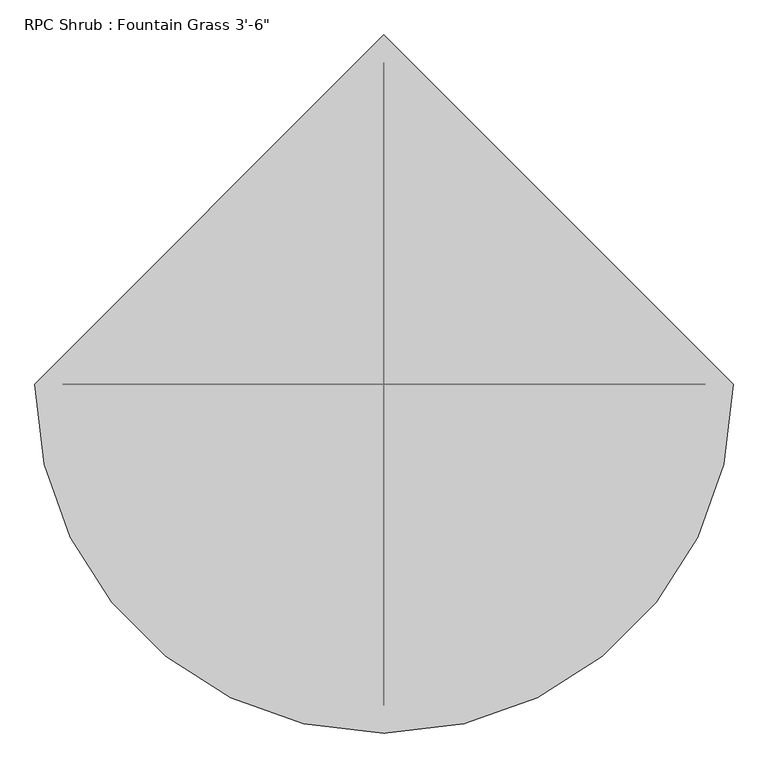
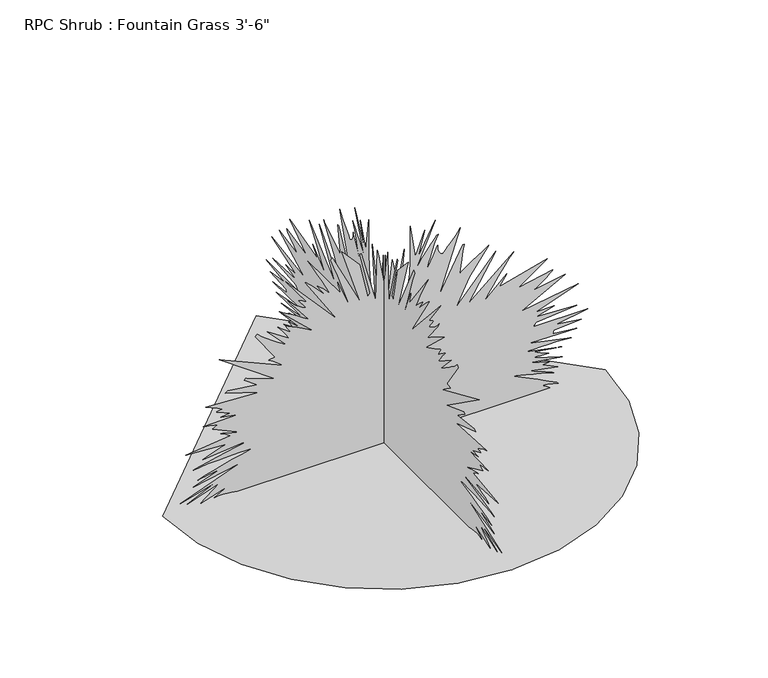
"""IFC4 building model written with IfcOpenShell, lengths in millimetres: geographic element geometry."""

from ifc_helpers import new_model, si_unit, origin, place, context, project, spatial, triangles, source, transform, mapped, element, save


def geographic_element_3d6ded1d(model_context):
    return source(origin(), model_context, "Body", "Tessellation", [
        triangles([(-1075.1021822, 0.0, 0.0), (-1046.6796438, -246.3421583, 0.0), (-965.7324045, -472.5690837, 0.0), (-838.7452429, -672.1950891, 0.0), (-672.1950891, -838.7452429, 0.0), (-472.5690837, -965.7324045, 0.0), (-246.341904, -1046.6796438, 0.0), (4.7e-05, -1075.1021822, 0.0), (246.3421583, -1046.6796438, 0.0), (472.5690837, -965.7324045, 0.0), (672.1950891, -838.7452429, 0.0), (838.7452429, -672.1950891, 0.0), (965.7324045, -472.5690837, 0.0), (1046.6796438, -246.341904, 0.0), (1075.1021822, 9.4e-05, 0.0), (-0.000141, 1075.1021822, 0.0), (-0.0002094, 151.7493584, 903.5253731), (-0.0002064, 197.8505688, 1023.5783649), (-0.0002098, 163.2745906, 893.9190554), (-0.000206, 247.7932689, 1057.1952084), (-0.0002115, 151.7493584, 831.4910345), (-0.0002109, 167.7051159, 857.3634378), (-0.0002104, 186.8993659, 885.4837418), (-0.0002098, 207.3806375, 913.5837708), (-0.0002093, 227.1984504, 939.3926605), (-0.0002089, 244.4013429, 960.6372213), (-0.0002086, 257.0401245, 975.0516758), (-0.0002085, 263.1615169, 980.3602907), (-0.0002094, 247.7267213, 943.5176268), (-0.0002103, 234.4486256, 908.2090988), (-0.0002111, 223.4664289, 876.1391087), (-0.0002118, 214.9206206, 848.9967247), (-0.0002123, 208.9511085, 828.4836599), (-0.0002127, 205.6989088, 816.294215), (-0.0002127, 205.3039292, 814.1250887), (-0.0002127, 208.3029104, 818.0239786), (-0.0002124, 216.0537091, 832.5501995), (-0.000212, 226.6881618, 853.6500017), (-0.0002116, 238.3378685, 877.271961), (-0.0002112, 249.1338665, 899.3648712), (-0.0002109, 257.207756, 915.8748373), (-0.0002107, 260.692645, 922.748037), (-0.0002103, 260.2582965, 906.3549242), (-0.0002103, 263.0522939, 893.568568), (-0.0002106, 267.949415, 883.9953152), (-0.0002111, 273.8345936, 877.2388962), (-0.0002116, 279.5876763, 872.9031143), (-0.000212, 284.0860209, 870.5917728), (-0.0002121, 286.2119994, 869.908457), (-0.0002118, 297.8807457, 886.1644415), (-0.0002115, 309.7933362, 900.0811066), (-0.0002113, 321.8837319, 912.8293837), (-0.0002111, 334.0884012, 925.5801315), (-0.0002109, 346.3388163, 939.504427), (-0.0002105, 358.5765141, 955.7731287), (-0.0002101, 370.7304234, 975.5571682), (-0.0002182, 267.0019983, 658.6111799), (-0.000213, 382.2543929, 884.3153538), (-0.0002131, 389.9378629, 884.3153538), (-0.0002137, 385.7570498, 861.6865025), (-0.0002144, 381.2002785, 835.410272), (-0.0002152, 376.6689054, 808.0824343), (-0.0002159, 372.5719171, 782.3039932), (-0.0002165, 369.305474, 760.6733368), (-0.0002169, 367.2760194, 745.7889982), (-0.0002171, 366.8873803, 740.2492201), (-0.0002169, 377.1819918, 749.4998909), (-0.0002168, 398.429096, 764.5798571), (-0.0002166, 426.0591682, 782.8856438), (-0.0002164, 455.5053723, 801.8137035), (-0.0002163, 482.19564, 818.763105), (-0.0002161, 501.5631351, 831.122743), (-0.0002161, 509.0332824, 836.294157), (-0.0002187, 412.9883454, 706.6349201), (-0.0002218, 347.6799408, 572.1725244), (-0.0002178, 543.6077345, 793.0735394), (-0.0002226, 409.1478822, 572.1725244), (-0.0002221, 630.0006443, 760.9578398), (-0.0002225, 607.1482965, 733.4877869), (-0.0002229, 581.7076618, 698.9640947), (-0.0002232, 555.6879564, 661.3112331), (-0.0002235, 531.0982146, 624.4456781), (-0.0002238, 509.9451453, 592.2867763), (-0.000224, 494.2377829, 568.7536923), (-0.0002241, 485.9827998, 557.7656639), (-0.0002226, 597.394713, 658.6111799), (-0.0002236, 558.9747108, 605.7868607), (-0.0002249, 793.3225067, 668.217425), (-0.000226, 651.1791481, 567.3694018), (-0.0002272, 820.215996, 600.9862453), (-0.0002273, 814.2901949, 595.3652584), (-0.0002274, 803.8635057, 586.2314046), (-0.0002276, 790.0737951, 574.7607748), (-0.0002278, 774.0693214, 562.1243005), (-0.0002279, 756.9878059, 549.4928767), (-0.000228, 739.9748909, 538.045138), (-0.0002281, 724.171059, 528.951943), (-0.0002293, 881.683901, 557.7656639), (-0.0002299, 666.5461607, 442.5132874), (-0.0002323, 943.1518787, 485.7338688), (-0.0002317, 735.6975357, 413.6995302), (-0.0002329, 827.8994659, 413.6995302), (-0.0002325, 739.5380716, 389.6889682), (-0.0002353, 935.4683361, 380.0852303), (-0.0002333, 739.5380716, 360.875211), (-0.0002334, 737.0615513, 358.3860097), (-0.0002334, 734.2345436, 355.2567312), (-0.0002335, 731.3236748, 351.8201314), (-0.0002335, 728.5931728, 348.4089297), (-0.0002336, 726.3148235, 345.3558457), (-0.0002336, 724.7527096, 342.9987222), (-0.0002337, 724.171059, 341.6677714), (-0.0002372, 989.2528439, 341.6677714), (-0.0002359, 835.5829359, 317.6571731), (-0.0002381, 958.5188187, 298.4471538), (-0.0002366, 824.0564592, 288.843434), (-0.000237, 820.215996, 274.4365736), (-0.0002389, 935.4683361, 260.0296949), (-0.0002357, 704.9635832, 264.8328356), (-0.0002397, 908.5748468, 221.6119818), (-0.0002392, 879.3065025, 224.4689658), (-0.0002387, 841.8263048, 226.3310433), (-0.0002381, 800.7671831, 227.3607588), (-0.0002376, 760.7622849, 227.7214381), (-0.0002371, 726.4494083, 227.5753896), (-0.0002368, 702.461701, 227.0854304), (-0.0002367, 693.4371065, 226.4143594), (-0.0002399, 862.4738817, 192.7990239), (-0.0002375, 720.3305958, 212.0077533), (-0.0002395, 801.079664, 180.0418811), (-0.0002393, 789.8198135, 180.8544223), (-0.0002391, 775.0700598, 181.8744909), (-0.0002389, 758.976638, 182.9049694), (-0.0002386, 743.6934866, 183.7490131), (-0.0002385, 731.3642973, 184.2100133), (-0.0002384, 724.1406103, 184.090889), (-0.0002384, 724.171059, 183.194523), (-0.0002416, 866.3169611, 139.9746865), (-0.0002388, 708.8040464, 163.9857935), (-0.0002409, 802.8830423, 135.5523002), (-0.0002408, 799.4514931, 134.831959), (-0.0002408, 794.1606823, 134.0915427), (-0.0002407, 787.8817778, 133.3391994), (-0.0002407, 781.4835491, 132.5827867), (-0.0002406, 775.8346207, 131.8306978), (-0.0002406, 771.8087036, 131.0902815), (-0.0002406, 770.2720242, 130.3701946), (-0.0002426, 843.2664785, 96.75485), (-0.0002398, 697.2953739, 122.86552), (-0.0002401, 707.9455233, 119.2147799), (-0.0002406, 727.4654074, 112.0362392), (-0.0002412, 752.0246641, 102.744419), (-0.0002418, 777.7954748, 92.7543584), (-0.0002424, 800.9424631, 83.4810781), (-0.0002428, 817.6404264, 76.3393719), (-0.000243, 824.0564592, 72.7440018), (-0.0002423, 793.2310152, 81.617738), (-0.0002416, 757.9402914, 91.2158803), (-0.0002408, 721.5396063, 100.7012479), (-0.0002401, 687.3868217, 109.2361467), (-0.0002395, 658.8372562, 115.9836545), (-0.0002392, 639.2462282, 120.1060682), (-0.000239, 631.9691288, 120.7659571), (-0.00024, 666.4089598, 103.8820858), (-0.0002411, 705.799288, 84.5753155), (-0.0002422, 746.4087278, 64.5205076), (-0.0002433, 784.498554, 45.3925509), (-0.0002442, 816.3297506, 28.8660546), (-0.0002449, 838.1686792, 16.6156986), (-0.0002452, 846.2788673, 10.3164533), (-0.0002449, 834.4653442, 14.1385651), (-0.0002446, 820.7849293, 17.3725156), (-0.0002444, 806.5482256, 20.018432), (-0.0002441, 793.0684525, 22.0761847), (-0.0002439, 781.6562857, 23.5461577), (-0.0002438, 773.6197123, 24.4280193), (-0.0002437, 770.2720242, 24.7219217), (-0.0002438, 772.6468792, 22.8719915), (-0.000244, 777.9732983, 19.2397436), (-0.0002442, 785.103023, 14.5784422), (-0.0002445, 792.8881582, 9.6414491), (-0.0002447, 800.1804457, 5.1824076), (-0.0002449, 805.8319902, 1.9544036), (-0.000245, 808.6894466, 0.7109504), (-0.0002248, -712.2762182, 7.55e-05), (-0.0002247, -716.251339, 1.888295), (-0.0002245, -727.0437761, 4.4398649), (-0.0002242, -742.9644613, 7.0367071), (-0.0002239, -762.3193119, 9.0605264), (-0.0002236, -783.416498, 9.8934675), (-0.0002233, -804.5594662, 8.9170168), (-0.0002232, -824.0564592, 5.5131917), (-0.0002229, -758.7480183, 43.9307805), (-0.0002224, -893.2079069, 0.7110012), (-0.0002215, -801.0059767, 72.7440018), (-0.000221, -954.6783554, 19.9198029), (-0.000221, -820.215996, 82.3482439), (-0.0002201, -989.2528439, 34.3262887), (-0.0002208, -701.1205765, 139.9746865), (-0.0002191, -927.7848661, 96.75485), (-0.0002194, -808.6894466, 139.9746865), (-0.0002193, -812.3292681, 139.9878942), (-0.0002192, -822.1235104, 138.9035673), (-0.0002191, -836.3982931, 136.9663127), (-0.000219, -853.4747217, 134.4199656), (-0.0002188, -871.6762997, 131.5086244), (-0.0002187, -889.3216616, 128.4766238), (-0.0002185, -904.7343836, 125.5680804), (-0.0002186, -893.5940025, 129.4418265), (-0.0002187, -867.1881289, 137.4656826), (-0.0002189, -829.5479118, 148.2962261), (-0.0002191, -784.7068262, 160.5885445), (-0.0002194, -736.7034336, 172.9992332), (-0.0002196, -689.5686653, 184.1843608), (-0.0002199, -647.3361414, 192.7990239), (-0.0002198, -647.3361414, 197.6011291), (-0.0002195, -670.2748575, 197.8660475), (-0.000219, -707.9862185, 197.3700022), (-0.0002184, -755.0320387, 196.1048178), (-0.0002178, -805.9742054, 194.0624097), (-0.0002172, -855.3746058, 191.2351477), (-0.0002168, -897.79004, 187.6151289), (-0.0002165, -927.7848661, 183.194523), (-0.0002165, -918.4681383, 186.3568118), (-0.0002167, -893.3831142, 192.5249491), (-0.0002169, -856.8325836, 200.7720656), (-0.0002172, -813.1090897, 210.171837), (-0.0002176, -766.5153494, 219.7974123), (-0.0002179, -721.3516817, 228.7219402), (-0.0002182, -681.9131006, 236.0185879), (-0.0002181, -681.9131006, 240.8209655), (-0.000216, -881.683901, 221.6119818), (-0.000216, -877.2592438, 223.6533724), (-0.000216, -864.5567488, 228.9396232), (-0.000216, -846.1366522, 236.2129074), (-0.0002161, -824.5568647, 244.2159255), (-0.0002161, -802.3750065, 251.6913958), (-0.0002162, -782.1465174, 257.3830178), (-0.0002164, -766.4315609, 260.0296949), (-0.0002133, -962.3618254, 274.4365736), (-0.0002155, -747.2215416, 298.4471538), (-0.0002154, -748.9690367, 300.212453), (-0.0002152, -753.6680231, 303.7532252), (-0.000215, -760.5209478, 308.3607565), (-0.0002147, -768.7124537, 313.3315287), (-0.0002145, -777.4449875, 317.9594075), (-0.0002143, -785.9107498, 321.5357517), (-0.0002141, -793.3021591, 323.3569342), (-0.0002142, -787.9021254, 322.9682951), (-0.0002145, -773.9448378, 319.7958507), (-0.0002149, -754.7907017, 314.8758748), (-0.0002153, -733.8001951, 309.2421344), (-0.0002157, -714.3387377, 303.9360992), (-0.0002161, -699.7641912, 299.9914817), (-0.0002162, -693.4371065, 298.4471538), (-0.0002125, -831.7399292, 360.875211), (-0.0002125, -830.7239302, 362.5795401), (-0.0002124, -827.9833271, 364.8223901), (-0.0002124, -823.9904022, 367.3496704), (-0.0002124, -819.2127142, 369.9125227), (-0.0002124, -814.1174583, 372.2544219), (-0.0002124, -809.1745914, 374.1289078), (-0.0002124, -804.8489834, 375.2820714), (-0.0002124, -807.681078, 376.3869822), (-0.0002122, -815.2883898, 378.2437366), (-0.000212, -826.3196205, 380.5906863), (-0.0002117, -839.4361164, 383.168763), (-0.0002115, -853.2892679, 385.7163909), (-0.0002112, -866.5404213, 387.9770087), (-0.000211, -877.8408943, 389.6889682), (-0.0002131, -712.6470531, 394.4920907), (-0.0002116, -793.3225067, 408.8989511), (-0.0002121, -743.3810783, 413.6995302), (-0.0002103, -812.5324533, 442.5132874), (-0.0002103, -811.3640654, 443.8569191), (-0.0002103, -808.2246494, 445.132023), (-0.0002103, -803.6476032, 446.2470712), (-0.0002104, -798.178969, 447.1106812), (-0.0002104, -792.3547606, 447.6364486), (-0.0002105, -786.7133898, 447.7354978), (-0.0002106, -781.7985008, 447.31641), (-0.0002105, -785.3392731, 449.5770278), (-0.0002102, -794.7525066, 454.4588882), (-0.0002098, -808.222106, 461.0349403), (-0.0002094, -823.9294321, 468.375517), (-0.000209, -840.0584621, 475.5561107), (-0.0002086, -854.7929552, 481.6521049), (-0.0002083, -866.3169611, 485.7338688), (-0.0002122, -605.078183, 471.3270083), (-0.0002084, -770.2720242, 524.1513276), (-0.0002083, -758.7480183, 533.7550655), (-0.0002108, -616.6021889, 514.5450826), (-0.0002087, -678.0700939, 557.7656639), (-0.0002085, -670.386624, 567.3694018), (-0.0002119, -528.2407219, 514.5450826), (-0.0002026, -801.0059767, 706.6349201), (-0.0002107, -493.6662698, 572.1725244), (-0.0002103, -502.7518707, 579.84077), (-0.0002099, -513.8160936, 588.6494983), (-0.0002095, -525.7210719, 597.7502872), (-0.0002091, -537.32883, 606.3024905), (-0.0002087, -547.4989941, 613.4576134), (-0.0002085, -555.0935886, 618.3700315), (-0.0002084, -558.9772542, 620.1936848), (-0.0002084, -557.3414892, 621.3672323), (-0.0002084, -553.1149303, 622.2358566), (-0.0002085, -547.2958088, 622.8886511), (-0.0002085, -540.8924569, 623.4067881), (-0.0002086, -534.9133161, 623.8742014), (-0.0002086, -530.3616317, 624.3770777), (-0.0002086, -528.2407219, 624.99688), (-0.0002032, -624.2856588, 764.2598185), (-0.000203, -616.6021889, 773.8661362), (-0.0002039, -593.2849711, 753.716276), (-0.0002049, -567.5725871, 733.8154558), (-0.0002058, -541.6163589, 715.1616526), (-0.0002066, -517.5625946, 698.7558226), (-0.0002072, -497.5601091, 685.596088), (-0.0002077, -483.7552105, 676.68326), (-0.0002079, -478.2992935, 673.0180767), (-0.0002038, -566.6607242, 769.062941), (-0.0002074, -459.0893106, 697.0286751), (-0.0002072, -461.8096387, 701.9384771), (-0.0002069, -466.5873631, 709.5711508), (-0.0002066, -473.2904423, 719.5050648), (-0.0002061, -481.786726, 731.3211313), (-0.0002056, -491.9467163, 744.6002626), (-0.000205, -503.6332486, 758.9207548), (-0.0002044, -516.7167523, 773.8661362), (-0.0002045, -513.2318996, 772.2836746), (-0.0002048, -504.2098123, 766.0124004), (-0.0002052, -491.8044648, 756.8075117), (-0.0002057, -478.1697593, 746.4290754), (-0.0002062, -465.4570905, 736.6373766), (-0.0002065, -455.8177806, 729.1875406), (-0.0002067, -451.4058043, 725.842396), (-0.0002064, -455.2462675, 731.5675552), (-0.0002062, -459.8665524, 738.7150841), (-0.0002059, -464.8017526, 746.5230377), (-0.0002056, -469.5794769, 754.2243118), (-0.0002053, -473.7349282, 761.0594324), (-0.0002051, -476.7956062, 766.2588243), (-0.000205, -478.2992935, 769.062941), (-0.0002053, -467.4382559, 763.1752916), (-0.0002059, -448.0021966, 753.3581583), (-0.0002066, -423.3616948, 740.947724), (-0.0002073, -396.8746124, 727.2876566), (-0.0002081, -371.9089851, 713.7214788), (-0.0002087, -351.8277617, 701.5879171), (-0.0002091, -339.9964345, 692.2280233), (-0.0002022, -509.0332824, 850.7010538), (-0.0002024, -501.3497761, 846.621797), (-0.000203, -481.4362023, 834.9479456), (-0.0002039, -453.9940547, 818.4430664), (-0.0002048, -423.7299863, 799.8731243), (-0.0002057, -395.3480704, 782.0093164), (-0.0002064, -373.5523441, 767.6151369), (-0.0002068, -363.0469171, 759.4592394), (-0.0002065, -368.546, 766.7414257), (-0.0002058, -383.526917, 785.5628059), (-0.0002047, -404.1618493, 811.3869564), (-0.0002036, -426.6281379, 839.67491), (-0.0002025, -447.1030509, 865.8851561), (-0.0002018, -461.7588424, 885.4786549), (-0.0002014, -466.7727805, 893.9190554), (-0.0002023, -448.2638449, 874.4677717), (-0.000203, -430.4813184, 858.5800787), (-0.0002036, -414.1669072, 846.0858559), (-0.000204, -400.0597741, 836.8173809), (-0.0002044, -388.9066395, 830.6070768), (-0.0002046, -381.4441226, 827.2873667), (-0.0002046, -378.4138933, 826.687912), (-0.0002027, -412.9883454, 874.7116522), (-0.0002028, -410.1994168, 874.6379648), (-0.0002029, -404.7105077, 872.2808413), (-0.0002031, -397.603565, 868.4733702), (-0.0002034, -389.9581741, 864.0537998), (-0.0002036, -382.8487244, 859.8627766), (-0.0002037, -377.3623587, 856.730991), (-0.0002038, -374.5708866, 855.5016329), (-0.0001983, -478.2992935, 994.7671148), (-0.0002099, -228.5847938, 716.2386217), (-0.0002007, -382.2543929, 956.3471489), (-0.0002008, -377.5401458, 953.682704), (-0.0002013, -366.727361, 944.1653343), (-0.0002019, -351.5610629, 929.5552523), (-0.0002027, -333.7912173, 911.6203005), (-0.0002035, -315.1705153, 892.1258509), (-0.0002043, -297.4463973, 872.8294996), (-0.000205, -282.3689745, 855.5016329), (-0.0002026, -324.6294582, 917.9296537), (-0.0002027, -320.6416566, 916.0831095), (-0.000203, -312.1021706, 909.1260487), (-0.0002035, -300.8906456, 898.981319), (-0.000204, -288.8891434, 887.5817968), (-0.0002045, -277.9849398, 876.8528732), (-0.0002048, -270.0626945, 868.7172506), (-0.000205, -267.0019983, 865.1053345), (-0.0002046, -271.2920526, 874.9732641), (-0.0002037, -283.4510124, 899.7559811), (-0.0002024, -300.8601605, 934.157733), (-0.000201, -320.9083554, 972.880006), (-0.0001996, -340.9768616, 1010.6243591), (-0.0001985, -358.4571536, 1042.097438), (-0.0001977, -370.7304234, 1061.9957874), (-0.0002064, -209.3757919, 841.0947361), (-0.0002061, -212.3376932, 849.9161453), (-0.0002058, -215.4885547, 860.5994322), (-0.0002054, -218.5616956, 872.0446638), (-0.000205, -221.2901628, 883.1571396), (-0.0002047, -223.4082747, 892.8396154), (-0.0002045, -224.6477885, 899.9947746), (-0.0002044, -224.7430407, 903.5253731), (-0.0002098, -163.2748449, 749.8529943), (-0.0002094, -166.4719427, 760.9984623), (-0.0002084, -175.9733068, 790.7926466), (-0.0002069, -190.101278, 833.7744707), (-0.0002052, -207.1779428, 884.4830034), (-0.0002033, -225.5248425, 937.4622551), (-0.0002016, -243.4645905, 987.2487511), (-0.0002002, -259.318492, 1028.3814875), (-0.0002, -251.6352582, 1037.9851891), (-0.0002099, -116.1998023, 765.6542828), (-0.0002002, -205.5340569, 1052.3920858), (-0.0002042, -117.1738889, 956.3471489), (-0.00021, -78.7561757, 778.6667152), (-0.00021, -77.3934682, 780.4573763), (-0.0002099, -75.5994689, 782.9009045), (-0.0002099, -73.577631, 785.6593117), (-0.0002098, -71.5275972, 788.3949005), (-0.0002098, -69.6525708, 790.7697556), (-0.0002097, -68.1529576, 792.4410925), (-0.0002097, -67.2306846, 793.0735394), (-0.0002026, -117.1738889, 1009.1714682), (-0.0002027, -109.4901464, 1009.1714682), (-0.0002115, -40.3384626, 745.0523426), (-0.000204, -32.6549699, 999.5677666), (-0.0002043, -30.2686421, 991.1984373), (-0.0002051, -25.7212838, 968.6636209), (-0.0002061, -19.6890689, 935.823983), (-0.0002074, -12.8482471, 896.5454212), (-0.0002087, -5.8757252, 854.6837322), (-0.00021, 0.5533969, 814.1047411), (-0.0002111, 5.7626445, 778.6667152), (-0.0002057, 5.7626445, 961.1502714), (-0.0002127, 17.2877302, 730.6455185), (-0.0002072, 40.3384626, 927.5359715), (-0.0002115, 67.2306846, 793.0735394), (-0.0002069, 97.9646508, 961.1502714), (-0.0002145, 74.9141773, 697.0286751), (-0.0002143, 99.6672177, 714.3946209), (-0.0002131, 115.3773507, 759.9418407), (-0.0002114, 124.0562722, 823.853274), (-0.0002092, 127.7161506, 896.3143307), (-0.0002071, 128.3684273, 967.5027906), (-0.0002053, 128.0255249, 1027.6042093), (-0.0002042, 128.6986215, 1066.79891), (151.7493584, -7.84e-05, 903.5253731), (197.8503144, -8.55e-05, 1023.5783649), (163.2745906, -7.78e-05, 893.9190554), (247.7932689, -8.75e-05, 1057.1952084), (151.7493584, -7.41e-05, 831.4910345), (167.7048616, -7.56e-05, 857.3634378), (186.8991115, -7.73e-05, 885.4837418), (207.3803832, -7.9e-05, 913.5837708), (227.1984504, -8.05e-05, 939.3901171), (244.4013429, -8.18e-05, 960.6372213), (257.0401245, -8.26e-05, 975.0516758), (263.1615169, -8.29e-05, 980.3602907), (247.726467, -8.07e-05, 943.5176268), (234.4483712, -7.86e-05, 908.2090988), (223.4661746, -7.67e-05, 876.1391087), (214.9203662, -7.51e-05, 848.9967247), (208.9508542, -7.39e-05, 828.4811165), (205.6986544, -7.32e-05, 816.294215), (205.3036749, -7.3e-05, 814.1250887), (208.3026561, -7.32e-05, 818.0239786), (216.0534548, -7.4e-05, 832.5501995), (226.6879074, -7.52e-05, 853.6500017), (238.3376142, -7.65e-05, 877.271961), (249.1336122, -7.77e-05, 899.3623278), (257.207756, -7.86e-05, 915.8748373), (260.692645, -7.9e-05, 922.748037), (260.2582965, -7.89e-05, 906.3549242), (263.0522939, -7.86e-05, 893.568568), (267.949415, -7.8e-05, 883.9953152), (273.8345936, -7.75e-05, 877.2388962), (279.5876763, -7.69e-05, 872.9031143), (284.0860209, -7.65e-05, 870.5917728), (286.2119994, -7.64e-05, 869.908457), (297.8807457, -7.73e-05, 886.1644415), (309.7933362, -7.82e-05, 900.0811066), (321.8837319, -7.89e-05, 912.8293837), (334.0884012, -7.97e-05, 925.5801315), (346.3388163, -8.05e-05, 939.504427), (358.5765141, -8.15e-05, 955.7731287), (370.7304234, -8.26e-05, 975.5571682), (267.0019983, -6.38e-05, 658.6111799), (382.2543929, -7.72e-05, 884.3153538), (389.9378629, -7.72e-05, 884.3153538), (385.7570498, -7.59e-05, 861.6865025), (381.2002785, -7.43e-05, 835.410272), (376.6689054, -7.27e-05, 808.0824343), (372.5693736, -7.11e-05, 782.3039932), (369.305474, -6.98e-05, 760.6733368), (367.2760194, -6.9e-05, 745.7889982), (366.8873803, -6.86e-05, 740.2492201), (377.1819918, -6.92e-05, 749.4998909), (398.429096, -7.01e-05, 764.5798571), (426.0591682, -7.12e-05, 782.8856438), (455.5053723, -7.23e-05, 801.8137035), (482.19564, -7.33e-05, 818.763105), (501.5631351, -7.4e-05, 831.122743), (509.0332824, -7.43e-05, 836.294157), (412.9883454, -6.66e-05, 706.6349201), (347.6799408, -5.86e-05, 572.1725244), (543.6077345, -7.18e-05, 793.0735394), (409.1478822, -5.86e-05, 572.1725244), (629.9981009, -6.77e-05, 760.9578398), (607.145753, -6.62e-05, 733.4877869), (581.7076618, -6.44e-05, 698.9640947), (555.6879564, -6.26e-05, 661.3112331), (531.0982146, -6.09e-05, 624.4456781), (509.9451453, -5.94e-05, 592.2867763), (494.2377829, -5.83e-05, 568.7536923), (485.9827998, -5.77e-05, 557.7656639), (597.3921696, -6.38e-05, 658.6111799), (558.9747108, -6.06e-05, 605.7868607), (793.3225067, -6.43e-05, 668.217425), (651.1791481, -5.83e-05, 567.3694018), (820.215996, -6.03e-05, 600.9862453), (814.2901949, -6e-05, 595.3652584), (803.8635057, -5.94e-05, 586.2314046), (790.0737951, -5.88e-05, 574.7607748), (774.0693214, -5.8e-05, 562.1243005), (756.9878059, -5.73e-05, 549.4928767), (739.9748909, -5.66e-05, 538.045138), (724.171059, -5.6e-05, 528.951943), (881.683901, -5.77e-05, 557.7656639), (666.5461607, -5.09e-05, 442.5132874), (943.1518787, -5.35e-05, 485.7338688), (735.6975357, -4.92e-05, 413.6995302), (827.8994659, -4.92e-05, 413.6995302), (739.5380716, -4.77e-05, 389.6889682), (935.4683361, -4.72e-05, 380.0852303), (739.5380716, -4.6e-05, 360.875211), (737.0615513, -4.59e-05, 358.3860097), (734.2345436, -4.57e-05, 355.2567312), (731.3236748, -4.55e-05, 351.8201314), (728.5931728, -4.53e-05, 348.4089297), (726.3148235, -4.51e-05, 345.3558457), (724.7527096, -4.49e-05, 342.9987222), (724.171059, -4.49e-05, 341.6677714), (989.2528439, -4.49e-05, 341.6677714), (835.5829359, -4.34e-05, 317.6571731), (958.5188187, -4.23e-05, 298.4471538), (824.0564592, -4.17e-05, 288.843434), (820.215996, -4.09e-05, 274.4365736), (935.4683361, -4e-05, 260.0296949), (704.9635832, -4.03e-05, 264.8328356), (908.5748468, -3.77e-05, 221.6119818), (879.3065025, -3.79e-05, 224.4689658), (841.8263048, -3.8e-05, 226.3310433), (800.7647123, -3.81e-05, 227.3607588), (760.7622849, -3.81e-05, 227.7211837), (726.4494083, -3.81e-05, 227.5753896), (702.461701, -3.8e-05, 227.0854304), (693.4371065, -3.8e-05, 226.4141051), (862.4738817, -3.6e-05, 192.7987696), (720.3305958, -3.71e-05, 212.007499), (801.079664, -3.52e-05, 180.0418811), (789.8198135, -3.53e-05, 180.8544223), (775.0700598, -3.53e-05, 181.8744909), (758.976638, -3.54e-05, 182.9049694), (743.6934866, -3.55e-05, 183.7490131), (731.3642973, -3.55e-05, 184.2100133), (724.1406103, -3.55e-05, 184.090889), (724.171059, -3.54e-05, 183.194523), (866.3169611, -3.28e-05, 139.9746865), (708.8040464, -3.43e-05, 163.9857935), (802.8830423, -3.26e-05, 135.5523002), (799.4514931, -3.25e-05, 134.831959), (794.1606823, -3.25e-05, 134.0915427), (787.8817778, -3.24e-05, 133.3391994), (781.4810057, -3.24e-05, 132.5827867), (775.8346207, -3.24e-05, 131.8306978), (771.8087036, -3.23e-05, 131.0902815), (770.2720242, -3.23e-05, 130.3701946), (843.2664785, -3.03e-05, 96.75485), (697.2953739, -3.18e-05, 122.8652657), (707.9455233, -3.16e-05, 119.2147799), (727.4654074, -3.12e-05, 112.0362392), (752.0246641, -3.06e-05, 102.744419), (777.7954748, -3e-05, 92.7543584), (800.9424631, -2.95e-05, 83.4810781), (817.6404264, -2.91e-05, 76.3393719), (824.0564592, -2.88e-05, 72.7440018), (793.2310152, -2.94e-05, 81.617738), (757.9402914, -2.99e-05, 91.2158803), (721.5396063, -3.05e-05, 100.7012479), (687.3868217, -3.1e-05, 109.2361467), (658.8372562, -3.14e-05, 115.9836545), (639.2462282, -3.17e-05, 120.1060682), (631.9691288, -3.17e-05, 120.7659571), (666.4089598, -3.07e-05, 103.8820858), (705.799288, -2.95e-05, 84.5753155), (746.4087278, -2.83e-05, 64.5205076), (784.498554, -2.72e-05, 45.3925509), (816.3297506, -2.62e-05, 28.8660546), (838.1686792, -2.55e-05, 16.6156986), (846.2788673, -2.51e-05, 10.3164533), (834.4653442, -2.53e-05, 14.1385651), (820.7849293, -2.55e-05, 17.3724907), (806.5482256, -2.57e-05, 20.018432), (793.0684525, -2.58e-05, 22.0761598), (781.6562857, -2.59e-05, 23.5461577), (773.6197123, -2.6e-05, 24.4280193), (770.2720242, -2.6e-05, 24.7219217), (772.6468792, -2.59e-05, 22.8719915), (777.9732983, -2.56e-05, 19.2397436), (785.103023, -2.54e-05, 14.5784422), (792.8881582, -2.51e-05, 9.6414491), (800.1804457, -2.48e-05, 5.1824076), (805.8319902, -2.46e-05, 1.9544036), (808.6894466, -2.45e-05, 0.7109504), (-712.2762182, -2.45e-05, 3.05e-05), (-716.251339, -2.46e-05, 1.8882493), (-727.0437761, -2.48e-05, 4.4398141), (-742.9644613, -2.49e-05, 7.0366566), (-762.3193119, -2.5e-05, 9.0604759), (-783.416498, -2.51e-05, 9.8934175), (-804.5594662, -2.5e-05, 8.9169657), (-824.0564592, -2.48e-05, 5.5131406), (-758.7480183, -2.71e-05, 43.9307805), (-893.2104504, -2.45e-05, 0.7109504), (-801.0059767, -2.88e-05, 72.7440018), (-954.6783554, -2.57e-05, 19.919753), (-820.215996, -2.94e-05, 82.3482439), (-989.2528439, -2.65e-05, 34.3262887), (-701.1205765, -3.28e-05, 139.9746865), (-927.7848661, -3.03e-05, 96.75485), (-808.6894466, -3.28e-05, 139.9746865), (-812.3292681, -3.28e-05, 139.9878942), (-822.1235104, -3.28e-05, 138.9035673), (-836.3982931, -3.27e-05, 136.9663127), (-853.4747217, -3.25e-05, 134.4197112), (-871.6762997, -3.23e-05, 131.5086244), (-889.3216616, -3.22e-05, 128.4766238), (-904.7343836, -3.2e-05, 125.5680804), (-893.5940025, -3.22e-05, 129.4418265), (-867.1881289, -3.27e-05, 137.4656826), (-829.5479118, -3.33e-05, 148.2959718), (-784.7068262, -3.41e-05, 160.5885445), (-736.7034336, -3.48e-05, 172.9992332), (-689.5686653, -3.55e-05, 184.1841064), (-647.3361414, -3.6e-05, 192.7987696), (-647.3361414, -3.63e-05, 197.6011291), (-670.2748575, -3.63e-05, 197.8660475), (-707.9862185, -3.63e-05, 197.3700022), (-755.0320387, -3.62e-05, 196.1045634), (-805.9767488, -3.61e-05, 194.0621554), (-855.3746058, -3.59e-05, 191.2351477), (-897.79004, -3.57e-05, 187.6151289), (-927.7848661, -3.54e-05, 183.194523), (-918.4681383, -3.56e-05, 186.3568118), (-893.3831142, -3.6e-05, 192.5249491), (-856.8325836, -3.65e-05, 200.7720656), (-813.1090897, -3.7e-05, 210.1715827), (-766.5153494, -3.76e-05, 219.797158), (-721.3516817, -3.81e-05, 228.7216859), (-681.9131006, -3.86e-05, 236.0185879), (-681.9131006, -3.89e-05, 240.8207112), (-881.683901, -3.77e-05, 221.6119818), (-877.2592438, -3.78e-05, 223.6533724), (-864.5567488, -3.81e-05, 228.9396232), (-846.1391956, -3.86e-05, 236.2129074), (-824.5568647, -3.91e-05, 244.2156711), (-802.3750065, -3.95e-05, 251.6913958), (-782.1465174, -3.98e-05, 257.3804744), (-766.4315609, -4e-05, 260.0296949), (-962.3618254, -4.09e-05, 274.4365736), (-747.2215416, -4.23e-05, 298.4471538), (-748.9690367, -4.24e-05, 300.212453), (-753.6705666, -4.26e-05, 303.7532252), (-760.5209478, -4.29e-05, 308.3607565), (-768.7149971, -4.32e-05, 313.3315287), (-777.4475309, -4.35e-05, 317.9594075), (-785.9107498, -4.37e-05, 321.5357517), (-793.3021591, -4.38e-05, 323.3569342), (-787.9021254, -4.38e-05, 322.9682951), (-773.9448378, -4.36e-05, 319.7958507), (-754.7907017, -4.33e-05, 314.8758748), (-733.8001951, -4.29e-05, 309.2421344), (-714.3387377, -4.26e-05, 303.9360992), (-699.7641912, -4.24e-05, 299.9914817), (-693.4371065, -4.23e-05, 298.4471538), (-831.7399292, -4.6e-05, 360.875211), (-830.7239302, -4.61e-05, 362.5795401), (-827.9833271, -4.62e-05, 364.8223901), (-823.9929457, -4.64e-05, 367.3496704), (-819.2127142, -4.66e-05, 369.9099792), (-814.1174583, -4.67e-05, 372.2544219), (-809.1745914, -4.68e-05, 374.1289078), (-804.8489834, -4.69e-05, 375.2820714), (-807.681078, -4.69e-05, 376.3869822), (-815.2883898, -4.7e-05, 378.2437366), (-826.3196205, -4.72e-05, 380.5906863), (-839.4361164, -4.73e-05, 383.168763), (-853.2918114, -4.75e-05, 385.7163909), (-866.5404213, -4.76e-05, 387.9770087), (-877.8408943, -4.77e-05, 389.6889682), (-712.6470531, -4.8e-05, 394.4920907), (-793.3225067, -4.89e-05, 408.8989511), (-743.3810783, -4.92e-05, 413.6995302), (-812.5324533, -5.09e-05, 442.5132874), (-811.3640654, -5.1e-05, 443.8569191), (-808.2246494, -5.1e-05, 445.132023), (-803.6501467, -5.11e-05, 446.2445277), (-798.178969, -5.12e-05, 447.1106812), (-792.3547606, -5.12e-05, 447.6364486), (-786.7133898, -5.12e-05, 447.7354978), (-781.7985008, -5.12e-05, 447.31641), (-785.3392731, -5.13e-05, 449.5770278), (-794.7525066, -5.16e-05, 454.4588882), (-808.222106, -5.2e-05, 461.0349403), (-823.9294321, -5.24e-05, 468.375517), (-840.0584621, -5.28e-05, 475.5561107), (-854.7929552, -5.32e-05, 481.6521049), (-866.3169611, -5.35e-05, 485.7338688), (-605.078183, -5.26e-05, 471.3270083), (-770.2720242, -5.57e-05, 524.1513276), (-758.7480183, -5.63e-05, 533.7550655), (-616.6021889, -5.52e-05, 514.5450826), (-678.0700939, -5.77e-05, 557.7656639), (-670.386624, -5.83e-05, 567.3694018), (-528.2432653, -5.52e-05, 514.5450826), (-801.0059767, -6.66e-05, 706.6349201), (-493.6662698, -5.86e-05, 572.1725244), (-502.7518707, -5.91e-05, 579.84077), (-513.8160936, -5.96e-05, 588.6494983), (-525.7210719, -6.01e-05, 597.7502872), (-537.32883, -6.06e-05, 606.3024905), (-547.4989941, -6.11e-05, 613.4576134), (-555.0935886, -6.14e-05, 618.3700315), (-558.9772542, -6.15e-05, 620.1936848), (-557.3440327, -6.15e-05, 621.3672323), (-553.1149303, -6.16e-05, 622.2358566), (-547.2958088, -6.16e-05, 622.8886511), (-540.8924569, -6.17e-05, 623.4042446), (-534.9133161, -6.17e-05, 623.8742014), (-530.3616317, -6.17e-05, 624.3770777), (-528.2432653, -6.18e-05, 624.99688), (-624.2856588, -7.01e-05, 764.2598185), (-616.6021889, -7.06e-05, 773.8635927), (-593.2849711, -6.94e-05, 753.716276), (-567.5725871, -6.82e-05, 733.8154558), (-541.6163589, -6.71e-05, 715.1616526), (-517.5625946, -6.62e-05, 698.7558226), (-497.5601091, -6.54e-05, 685.596088), (-483.7552105, -6.48e-05, 676.68326), (-478.2992935, -6.46e-05, 673.0180767), (-566.6607242, -7.03e-05, 769.062941), (-459.091854, -6.6e-05, 697.0286751), (-461.8096387, -6.63e-05, 701.9384771), (-466.5873631, -6.68e-05, 709.5711508), (-473.2904423, -6.74e-05, 719.5050648), (-481.786726, -6.81e-05, 731.3211313), (-491.9467163, -6.89e-05, 744.6002626), (-503.6332486, -6.97e-05, 758.9207548), (-516.7167523, -7.06e-05, 773.8635927), (-513.2318996, -7.05e-05, 772.2836746), (-504.2098123, -7.02e-05, 766.0124004), (-491.8044648, -6.96e-05, 756.8075117), (-478.1697593, -6.9e-05, 746.4290754), (-465.4570905, -6.84e-05, 736.6373766), (-455.8177806, -6.8e-05, 729.1875406), (-451.4058043, -6.78e-05, 725.842396), (-455.2462675, -6.81e-05, 731.5675552), (-459.8665524, -6.85e-05, 738.7150841), (-464.8017526, -6.9e-05, 746.5230377), (-469.5794769, -6.95e-05, 754.2243118), (-473.7349282, -6.99e-05, 761.0594324), (-476.7981497, -7.02e-05, 766.2588243), (-478.2992935, -7.03e-05, 769.062941), (-467.4382559, -7e-05, 763.1752916), (-448.0021966, -6.94e-05, 753.3581583), (-423.3616948, -6.87e-05, 740.947724), (-396.8746124, -6.79e-05, 727.2876566), (-371.9089851, -6.7e-05, 713.7214788), (-351.8277617, -6.63e-05, 701.5879171), (-339.9964345, -6.58e-05, 692.2280233), (-509.0332824, -7.52e-05, 850.7010538), (-501.3497761, -7.5e-05, 846.621797), (-481.4362023, -7.43e-05, 834.9479456), (-453.9940547, -7.33e-05, 818.4430664), (-423.7299863, -7.22e-05, 799.8731243), (-395.3480704, -7.11e-05, 782.0093164), (-373.5523441, -7.03e-05, 767.6151369), (-363.0469171, -6.98e-05, 759.4592394), (-368.546, -7.02e-05, 766.7414257), (-383.526917, -7.13e-05, 785.5628059), (-404.1618493, -7.29e-05, 811.3869564), (-426.6281379, -7.46e-05, 839.67491), (-447.1030509, -7.61e-05, 865.8851561), (-461.7588424, -7.73e-05, 885.4786549), (-466.7727805, -7.78e-05, 893.9190554), (-448.2638449, -7.66e-05, 874.4677717), (-430.4813184, -7.57e-05, 858.5800787), (-414.1669072, -7.49e-05, 846.0858559), (-400.0623176, -7.44e-05, 836.8173809), (-388.9066395, -7.4e-05, 830.6070768), (-381.4441226, -7.38e-05, 827.2873667), (-378.4138933, -7.38e-05, 826.687912), (-412.9883454, -7.66e-05, 874.7116522), (-410.1994168, -7.66e-05, 874.6379648), (-404.7105077, -7.65e-05, 872.2808413), (-397.603565, -7.63e-05, 868.4733702), (-389.9581741, -7.6e-05, 864.0537998), (-382.8487244, -7.58e-05, 859.8627766), (-377.3623587, -7.56e-05, 856.730991), (-374.5708866, -7.55e-05, 855.5016329), (-478.2992935, -8.38e-05, 994.7671148), (-228.5850482, -6.72e-05, 716.2386217), (-382.2543929, -8.15e-05, 956.3471489), (-377.5401458, -8.13e-05, 953.682704), (-366.727361, -8.08e-05, 944.1653343), (-351.5610629, -7.99e-05, 929.5552523), (-333.7912173, -7.88e-05, 911.6203005), (-315.1730587, -7.77e-05, 892.1258509), (-297.4463973, -7.65e-05, 872.8294996), (-282.3689745, -7.55e-05, 855.5016329), (-324.6294582, -7.92e-05, 917.9296537), (-320.6442, -7.91e-05, 916.0831095), (-312.1021706, -7.87e-05, 909.1260487), (-300.8906456, -7.81e-05, 898.981319), (-288.8891434, -7.74e-05, 887.5817968), (-277.9874833, -7.68e-05, 876.8528732), (-270.0626945, -7.63e-05, 868.7172506), (-267.0019983, -7.61e-05, 865.1053345), (-271.2920526, -7.67e-05, 874.9732641), (-283.4510124, -7.81e-05, 899.7559811), (-300.8601605, -8.02e-05, 934.157733), (-320.9083554, -8.25e-05, 972.880006), (-340.9768616, -8.47e-05, 1010.6243591), (-358.4571536, -8.66e-05, 1042.097438), (-370.7304234, -8.78e-05, 1061.9957874), (-209.3760462, -7.46e-05, 841.0947361), (-212.3379476, -7.52e-05, 849.9161453), (-215.4885547, -7.58e-05, 860.5994322), (-218.5616956, -7.65e-05, 872.0446638), (-221.2904171, -7.71e-05, 883.1571396), (-223.4082747, -7.77e-05, 892.8396154), (-224.6480428, -7.81e-05, 899.9947746), (-224.7430407, -7.84e-05, 903.5253731), (-163.2750993, -6.92e-05, 749.8529943), (-166.4719427, -6.99e-05, 760.9984623), (-175.9735611, -7.16e-05, 790.7901031), (-190.1015323, -7.42e-05, 833.7719273), (-207.1779428, -7.72e-05, 884.4830034), (-225.5250968, -8.04e-05, 937.4622551), (-243.4648448, -8.33e-05, 987.2487511), (-259.318492, -8.58e-05, 1028.3814875), (-251.6355125, -8.64e-05, 1037.9851891), (-116.2000566, -7.01e-05, 765.6542828), (-205.5343112, -8.72e-05, 1052.3920858), (-117.1738889, -8.15e-05, 956.3471489), (-78.7564301, -7.09e-05, 778.6667152), (-77.3934682, -7.1e-05, 780.4573763), (-75.5999776, -7.12e-05, 782.9009045), (-73.5778853, -7.13e-05, 785.6593117), (-71.5278515, -7.15e-05, 788.3949005), (-69.6528251, -7.16e-05, 790.7697556), (-68.1529576, -7.17e-05, 792.4410925), (-67.2311933, -7.18e-05, 793.0735394), (-117.1738889, -8.47e-05, 1009.1714682), (-109.4904008, -8.47e-05, 1009.1714682), (-40.3384626, -6.89e-05, 745.0523426), (-32.6552242, -8.41e-05, 999.5677666), (-30.2688964, -8.36e-05, 991.1984373), (-25.7212838, -8.22e-05, 968.6636209), (-19.6892211, -8.03e-05, 935.823983), (-12.8484243, -7.79e-05, 896.5454212), (-5.8759029, -7.54e-05, 854.6837322), (0.5532267, -7.3e-05, 814.1047411), (5.7624668, -7.09e-05, 778.6667152), (5.7624668, -8.18e-05, 961.1502714), (17.2875781, -6.81e-05, 730.6455185), (40.3382082, -7.98e-05, 927.5359715), (67.2306846, -7.18e-05, 793.0735394), (97.9646508, -8.18e-05, 961.1502714), (74.9141773, -6.6e-05, 697.0286751), (99.6669633, -6.71e-05, 714.3946209), (115.3770963, -6.98e-05, 759.9418407), (124.0560179, -7.36e-05, 823.853274), (127.7158962, -7.79e-05, 896.3143307), (128.3679186, -8.22e-05, 967.5027906), (128.0250162, -8.58e-05, 1027.6042093), (128.6986215, -8.81e-05, 1066.79891)], [[15, 16, 1], [14, 15, 1], [14, 1, 2], [13, 14, 2], [13, 2, 3], [13, 3, 4], [12, 13, 4], [11, 12, 4], [11, 4, 5], [11, 5, 6], [11, 6, 7], [11, 7, 8], [11, 8, 9], [11, 9, 10], [127, 128, 129], [197, 198, 199], [444, 445, 446], [117, 118, 119], [404, 405, 406], [19, 20, 21], [195, 196, 197], [119, 120, 121], [380, 381, 382], [448, 449, 450], [137, 138, 139], [103, 104, 105], [207, 208, 209], [112, 113, 114], [17, 18, 19], [199, 200, 201], [247, 248, 249], [403, 404, 406], [119, 121, 122], [269, 270, 271], [99, 100, 101], [222, 223, 224], [222, 224, 225], [239, 240, 241], [77, 78, 79], [268, 269, 271], [295, 296, 297], [114, 115, 116], [402, 403, 406], [75, 76, 77], [155, 156, 157], [154, 155, 157], [267, 268, 271], [456, 457, 17], [119, 122, 123], [85, 86, 87], [147, 148, 149], [101, 102, 103], [271, 272, 273], [320, 321, 322], [266, 267, 271], [455, 456, 17], [287, 288, 289], [364, 365, 366], [401, 402, 406], [363, 364, 366], [350, 351, 352], [350, 352, 353], [350, 353, 354], [77, 79, 80], [129, 130, 131], [97, 98, 99], [265, 266, 271], [55, 56, 57], [350, 354, 355], [231, 232, 233], [231, 233, 234], [231, 234, 235], [231, 235, 236], [231, 236, 237], [286, 287, 289], [129, 131, 132], [231, 237, 238], [231, 238, 239], [119, 123, 124], [191, 192, 193], [169, 170, 171], [87, 88, 89], [193, 194, 195], [72, 73, 74], [264, 265, 271], [400, 401, 406], [77, 80, 81], [285, 286, 289], [350, 355, 356], [183, 184, 185], [247, 249, 250], [246, 247, 250], [129, 132, 133], [284, 285, 289], [71, 72, 74], [436, 437, 438], [436, 438, 439], [436, 439, 440], [436, 440, 441], [54, 55, 57], [446, 447, 448], [328, 329, 330], [328, 330, 331], [139, 140, 141], [139, 141, 142], [139, 142, 143], [139, 143, 144], [283, 284, 289], [207, 209, 210], [206, 207, 210], [77, 81, 82], [350, 356, 357], [436, 441, 442], [182, 183, 185], [412, 413, 414], [411, 412, 414], [410, 411, 414], [409, 410, 414], [408, 409, 414], [407, 408, 414], [406, 407, 414], [139, 144, 145], [454, 455, 17], [70, 71, 74], [263, 264, 271], [399, 400, 406], [181, 182, 185], [282, 283, 289], [382, 383, 384], [382, 384, 385], [382, 385, 386], [382, 386, 387], [382, 387, 388], [382, 388, 389], [382, 389, 390], [180, 181, 185], [27, 28, 29], [26, 27, 29], [423, 424, 425], [423, 425, 426], [179, 180, 185], [89, 90, 91], [89, 91, 92], [89, 92, 93], [119, 124, 125], [53, 54, 57], [129, 133, 134], [153, 154, 157], [153, 157, 158], [152, 153, 158], [350, 357, 358], [178, 179, 185], [190, 191, 193], [139, 145, 146], [390, 391, 392], [390, 392, 393], [390, 393, 394], [390, 394, 395], [89, 93, 94], [41, 42, 43], [77, 82, 83], [89, 94, 95], [281, 282, 289], [177, 178, 185], [436, 442, 443], [52, 53, 57], [342, 343, 344], [69, 70, 74], [51, 52, 57], [50, 51, 57], [49, 50, 57], [89, 95, 96], [390, 395, 396], [221, 222, 225], [221, 225, 226], [398, 399, 406], [341, 342, 344], [205, 206, 210], [205, 210, 211], [204, 205, 211], [89, 96, 97], [77, 83, 84], [129, 134, 135], [195, 197, 199], [139, 146, 147], [139, 147, 149], [363, 366, 367], [362, 363, 367], [362, 367, 368], [152, 158, 159], [151, 152, 159], [245, 246, 250], [245, 250, 251], [244, 245, 251], [203, 204, 211], [372, 373, 374], [372, 374, 375], [372, 375, 376], [372, 376, 377], [372, 377, 378], [436, 443, 444], [289, 290, 291], [289, 291, 292], [77, 84, 85], [189, 190, 193], [68, 69, 74], [303, 304, 305], [446, 448, 450], [168, 169, 171], [168, 171, 172], [40, 41, 43], [328, 331, 332], [327, 328, 332], [119, 125, 126], [168, 172, 173], [372, 378, 379], [303, 305, 306], [193, 195, 199], [203, 211, 212], [202, 203, 212], [201, 202, 212], [199, 201, 212], [199, 212, 213], [199, 213, 214], [167, 168, 173], [167, 173, 174], [25, 26, 29], [25, 29, 30], [167, 174, 175], [327, 332, 333], [326, 327, 333], [24, 25, 30], [273, 274, 275], [273, 275, 276], [273, 276, 277], [273, 277, 278], [273, 278, 279], [273, 279, 280], [273, 280, 281], [273, 281, 289], [271, 273, 289], [129, 135, 136], [390, 396, 397], [361, 362, 368], [361, 368, 369], [340, 341, 344], [231, 239, 241], [243, 244, 251], [243, 251, 252], [242, 243, 252], [241, 242, 252], [231, 241, 252], [231, 252, 253], [231, 253, 254], [231, 254, 255], [89, 97, 99], [372, 379, 380], [372, 380, 382], [255, 256, 257], [255, 257, 258], [255, 258, 259], [255, 259, 260], [255, 260, 261], [255, 261, 262], [255, 262, 263], [255, 263, 271], [112, 114, 116], [150, 151, 159], [150, 159, 160], [149, 150, 160], [433, 434, 435], [433, 435, 436], [292, 293, 294], [292, 294, 295], [289, 292, 295], [326, 333, 334], [325, 326, 334], [24, 30, 31], [23, 24, 31], [436, 444, 446], [421, 422, 423], [420, 421, 423], [419, 420, 423], [418, 419, 423], [417, 418, 423], [416, 417, 423], [415, 416, 423], [414, 415, 423], [58, 59, 60], [57, 58, 60], [57, 60, 61], [57, 61, 62], [57, 62, 63], [57, 63, 64], [57, 64, 65], [57, 65, 66], [361, 369, 370], [67, 68, 74], [40, 43, 44], [23, 31, 32], [22, 23, 32], [22, 32, 33], [340, 344, 345], [339, 340, 345], [338, 339, 345], [302, 303, 306], [302, 306, 307], [188, 189, 193], [325, 334, 335], [324, 325, 335], [221, 226, 227], [220, 221, 227], [220, 227, 228], [219, 220, 228], [219, 228, 229], [218, 219, 229], [218, 229, 230], [217, 218, 230], [360, 361, 370], [360, 370, 371], [360, 371, 372], [360, 372, 382], [359, 360, 382], [358, 359, 382], [350, 358, 382], [324, 335, 336], [323, 324, 336], [167, 175, 176], [166, 167, 176], [166, 176, 177], [166, 177, 185], [165, 166, 185], [164, 165, 185], [163, 164, 185], [311, 312, 313], [311, 313, 314], [311, 314, 315], [311, 315, 316], [311, 316, 317], [311, 317, 318], [112, 116, 117], [112, 117, 119], [311, 318, 319], [302, 307, 308], [301, 302, 308], [301, 308, 309], [337, 338, 345], [337, 345, 346], [336, 337, 346], [390, 397, 398], [382, 390, 398], [382, 398, 406], [382, 406, 414], [432, 433, 436], [431, 432, 436], [430, 431, 436], [429, 430, 436], [428, 429, 436], [427, 428, 436], [426, 427, 436], [48, 49, 57], [119, 126, 127], [21, 22, 33], [21, 33, 34], [21, 34, 35], [66, 67, 74], [66, 74, 75], [57, 66, 75], [39, 40, 44], [39, 44, 45], [301, 309, 310], [300, 301, 310], [300, 310, 311], [255, 271, 289], [47, 48, 57], [453, 454, 17], [453, 17, 19], [453, 19, 21], [311, 319, 320], [216, 217, 230], [452, 453, 21], [452, 21, 35], [188, 193, 199], [187, 188, 199], [186, 187, 199], [185, 186, 199], [163, 185, 199], [163, 199, 214], [163, 214, 215], [163, 215, 216], [322, 323, 336], [46, 47, 57], [87, 89, 99], [85, 87, 99], [99, 101, 103], [99, 103, 105], [99, 105, 106], [99, 106, 107], [99, 107, 108], [99, 108, 109], [99, 109, 110], [99, 110, 111], [99, 111, 112], [300, 311, 320], [299, 300, 320], [298, 299, 320], [297, 298, 320], [149, 160, 161], [139, 149, 161], [127, 129, 136], [99, 112, 119], [39, 45, 46], [39, 46, 57], [38, 39, 57], [37, 38, 57], [36, 37, 57], [35, 36, 57], [452, 35, 57], [451, 452, 57], [423, 426, 436], [216, 230, 231], [322, 336, 346], [322, 346, 347], [85, 99, 119], [85, 119, 127], [136, 137, 139], [127, 136, 139], [127, 139, 161], [127, 161, 162], [85, 127, 162], [85, 162, 163], [85, 163, 216], [77, 85, 216], [75, 77, 216], [57, 75, 216], [57, 216, 231], [57, 231, 255], [57, 255, 289], [57, 289, 295], [57, 295, 297], [57, 297, 320], [57, 320, 322], [322, 347, 348], [450, 451, 57], [322, 348, 349], [322, 349, 350], [57, 322, 350], [450, 57, 350], [450, 350, 382], [446, 450, 382], [436, 446, 382], [436, 382, 414], [423, 436, 414], [568, 569, 570], [638, 639, 640], [885, 886, 887], [558, 559, 560], [845, 846, 847], [460, 461, 462], [636, 637, 638], [560, 561, 562], [821, 822, 823], [889, 890, 891], [578, 579, 580], [544, 545, 546], [648, 649, 650], [553, 554, 555], [458, 459, 460], [640, 641, 642], [688, 689, 690], [844, 845, 847], [560, 562, 563], [710, 711, 712], [540, 541, 542], [663, 664, 665], [663, 665, 666], [680, 681, 682], [518, 519, 520], [709, 710, 712], [736, 737, 738], [555, 556, 557], [843, 844, 847], [516, 517, 518], [596, 597, 598], [595, 596, 598], [708, 709, 712], [897, 898, 458], [560, 563, 564], [526, 527, 528], [588, 589, 590], [542, 543, 544], [712, 713, 714], [761, 762, 763], [707, 708, 712], [896, 897, 458], [728, 729, 730], [805, 806, 807], [842, 843, 847], [804, 805, 807], [791, 792, 793], [791, 793, 794], [791, 794, 795], [518, 520, 521], [570, 571, 572], [538, 539, 540], [706, 707, 712], [496, 497, 498], [791, 795, 796], [672, 673, 674], [672, 674, 675], [672, 675, 676], [672, 676, 677], [672, 677, 678], [727, 728, 730], [570, 572, 573], [672, 678, 679], [672, 679, 680], [560, 564, 565], [632, 633, 634], [610, 611, 612], [528, 529, 530], [634, 635, 636], [513, 514, 515], [705, 706, 712], [841, 842, 847], [518, 521, 522], [726, 727, 730], [791, 796, 797], [624, 625, 626], [688, 690, 691], [687, 688, 691], [570, 573, 574], [725, 726, 730], [512, 513, 515], [877, 878, 879], [877, 879, 880], [877, 880, 881], [877, 881, 882], [495, 496, 498], [887, 888, 889], [769, 770, 771], [769, 771, 772], [580, 581, 582], [580, 582, 583], [580, 583, 584], [580, 584, 585], [724, 725, 730], [648, 650, 651], [647, 648, 651], [518, 522, 523], [791, 797, 798], [877, 882, 883], [623, 624, 626], [853, 854, 855], [852, 853, 855], [851, 852, 855], [850, 851, 855], [849, 850, 855], [848, 849, 855], [847, 848, 855], [580, 585, 586], [895, 896, 458], [511, 512, 515], [704, 705, 712], [840, 841, 847], [622, 623, 626], [723, 724, 730], [823, 824, 825], [823, 825, 826], [823, 826, 827], [823, 827, 828], [823, 828, 829], [823, 829, 830], [823, 830, 831], [621, 622, 626], [468, 469, 470], [467, 468, 470], [864, 865, 866], [864, 866, 867], [620, 621, 626], [530, 531, 532], [530, 532, 533], [530, 533, 534], [560, 565, 566], [494, 495, 498], [570, 574, 575], [594, 595, 598], [594, 598, 599], [593, 594, 599], [791, 798, 799], [619, 620, 626], [631, 632, 634], [580, 586, 587], [831, 832, 833], [831, 833, 834], [831, 834, 835], [831, 835, 836], [530, 534, 535], [482, 483, 484], [518, 523, 524], [530, 535, 536], [722, 723, 730], [618, 619, 626], [877, 883, 884], [493, 494, 498], [783, 784, 785], [510, 511, 515], [492, 493, 498], [491, 492, 498], [490, 491, 498], [530, 536, 537], [831, 836, 837], [662, 663, 666], [662, 666, 667], [839, 840, 847], [782, 783, 785], [646, 647, 651], [646, 651, 652], [645, 646, 652], [530, 537, 538], [518, 524, 525], [570, 575, 576], [636, 638, 640], [580, 587, 588], [580, 588, 590], [804, 807, 808], [803, 804, 808], [803, 808, 809], [593, 599, 600], [592, 593, 600], [686, 687, 691], [686, 691, 692], [685, 686, 692], [644, 645, 652], [813, 814, 815], [813, 815, 816], [813, 816, 817], [813, 817, 818], [813, 818, 819], [877, 884, 885], [730, 731, 732], [730, 732, 733], [518, 525, 526], [630, 631, 634], [509, 510, 515], [744, 745, 746], [887, 889, 891], [609, 610, 612], [609, 612, 613], [481, 482, 484], [769, 772, 773], [768, 769, 773], [560, 566, 567], [609, 613, 614], [813, 819, 820], [744, 746, 747], [634, 636, 640], [644, 652, 653], [643, 644, 653], [642, 643, 653], [640, 642, 653], [640, 653, 654], [640, 654, 655], [608, 609, 614], [608, 614, 615], [466, 467, 470], [466, 470, 471], [608, 615, 616], [768, 773, 774], [767, 768, 774], [465, 466, 471], [714, 715, 716], [714, 716, 717], [714, 717, 718], [714, 718, 719], [714, 719, 720], [714, 720, 721], [714, 721, 722], [714, 722, 730], [712, 714, 730], [570, 576, 577], [831, 837, 838], [802, 803, 809], [802, 809, 810], [781, 782, 785], [672, 680, 682], [684, 685, 692], [684, 692, 693], [683, 684, 693], [682, 683, 693], [672, 682, 693], [672, 693, 694], [672, 694, 695], [672, 695, 696], [530, 538, 540], [813, 820, 821], [813, 821, 823], [696, 697, 698], [696, 698, 699], [696, 699, 700], [696, 700, 701], [696, 701, 702], [696, 702, 703], [696, 703, 704], [696, 704, 712], [553, 555, 557], [591, 592, 600], [591, 600, 601], [590, 591, 601], [874, 875, 876], [874, 876, 877], [733, 734, 735], [733, 735, 736], [730, 733, 736], [767, 774, 775], [766, 767, 775], [465, 471, 472], [464, 465, 472], [877, 885, 887], [862, 863, 864], [861, 862, 864], [860, 861, 864], [859, 860, 864], [858, 859, 864], [857, 858, 864], [856, 857, 864], [855, 856, 864], [499, 500, 501], [498, 499, 501], [498, 501, 502], [498, 502, 503], [498, 503, 504], [498, 504, 505], [498, 505, 506], [498, 506, 507], [802, 810, 811], [508, 509, 515], [481, 484, 485], [464, 472, 473], [463, 464, 473], [463, 473, 474], [781, 785, 786], [780, 781, 786], [779, 780, 786], [743, 744, 747], [743, 747, 748], [629, 630, 634], [766, 775, 776], [765, 766, 776], [662, 667, 668], [661, 662, 668], [661, 668, 669], [660, 661, 669], [660, 669, 670], [659, 660, 670], [659, 670, 671], [658, 659, 671], [801, 802, 811], [801, 811, 812], [801, 812, 813], [801, 813, 823], [800, 801, 823], [799, 800, 823], [791, 799, 823], [765, 776, 777], [764, 765, 777], [608, 616, 617], [607, 608, 617], [607, 617, 618], [607, 618, 626], [606, 607, 626], [605, 606, 626], [604, 605, 626], [752, 753, 754], [752, 754, 755], [752, 755, 756], [752, 756, 757], [752, 757, 758], [752, 758, 759], [553, 557, 558], [553, 558, 560], [752, 759, 760], [743, 748, 749], [742, 743, 749], [742, 749, 750], [778, 779, 786], [778, 786, 787], [777, 778, 787], [831, 838, 839], [823, 831, 839], [823, 839, 847], [823, 847, 855], [873, 874, 877], [872, 873, 877], [871, 872, 877], [870, 871, 877], [869, 870, 877], [868, 869, 877], [867, 868, 877], [489, 490, 498], [560, 567, 568], [462, 463, 474], [462, 474, 475], [462, 475, 476], [507, 508, 515], [507, 515, 516], [498, 507, 516], [480, 481, 485], [480, 485, 486], [742, 750, 751], [741, 742, 751], [741, 751, 752], [696, 712, 730], [488, 489, 498], [894, 895, 458], [894, 458, 460], [894, 460, 462], [752, 760, 761], [657, 658, 671], [893, 894, 462], [893, 462, 476], [629, 634, 640], [628, 629, 640], [627, 628, 640], [626, 627, 640], [604, 626, 640], [604, 640, 655], [604, 655, 656], [604, 656, 657], [763, 764, 777], [487, 488, 498], [528, 530, 540], [526, 528, 540], [540, 542, 544], [540, 544, 546], [540, 546, 547], [540, 547, 548], [540, 548, 549], [540, 549, 550], [540, 550, 551], [540, 551, 552], [540, 552, 553], [741, 752, 761], [740, 741, 761], [739, 740, 761], [738, 739, 761], [590, 601, 602], [580, 590, 602], [568, 570, 577], [540, 553, 560], [480, 486, 487], [480, 487, 498], [479, 480, 498], [478, 479, 498], [477, 478, 498], [476, 477, 498], [893, 476, 498], [892, 893, 498], [864, 867, 877], [657, 671, 672], [763, 777, 787], [763, 787, 788], [526, 540, 560], [526, 560, 568], [577, 578, 580], [568, 577, 580], [568, 580, 602], [568, 602, 603], [526, 568, 603], [526, 603, 604], [526, 604, 657], [518, 526, 657], [516, 518, 657], [498, 516, 657], [498, 657, 672], [498, 672, 696], [498, 696, 730], [498, 730, 736], [498, 736, 738], [498, 738, 761], [498, 761, 763], [763, 788, 789], [891, 892, 498], [763, 789, 790], [763, 790, 791], [498, 763, 791], [891, 498, 791], [891, 791, 823], [887, 891, 823], [877, 887, 823], [877, 823, 855], [864, 877, 855]], closed=False),
    ])


if __name__ == "__main__":
    model = new_model("IFC4")
    model_context = context("Model", 3, world=origin())
    ifc_project = project(units=[si_unit("LENGTHUNIT", "METRE", prefix="MILLI")], contexts=[model_context])
    site = spatial("IfcSite", under=ifc_project)
    building = spatial("IfcBuilding", under=site)
    placement = place(None, origin())
    geographic_element_shape = geographic_element_3d6ded1d(model_context)
    element("IfcGeographicElement", 1, ObjectType="RPC Shrub : Fountain Grass 3'-6\"", at=placement, inside=building, context=model_context, shape_type="MappedRepresentation", body=[
        mapped(geographic_element_shape, transform((0.0, 0.0, 0.0), x_axis=(1.0, 0.0, 0.0), y_axis=(0.0, 1.0, 0.0), z_axis=(0.0, 0.0, 1.0))),
    ])
    save(model, "model.ifc")

# Revit data of these elements
# Type "RPC Shrub : Fountain Grass 3'-6\""
#   Type Comments = "Fountain Grass"
#   built-in parameter 1005198 = "{2, 15},{39, RPC-16-G1GP-21FX-7KGL-L000-ST1L-LVER-AU},{1, 0},{1, 0},{2, 13},{1, 8},{5, Color},{1, 0},{1, 0},{3, 0.8},{3, 0.8},{3, 0.8},{1, 8},{7, BBoxMin},{1, 0},{1, 0},{1, 0},{1, 0},{1, 0},{1, 8},{7, BBoxMax},{1, 0},{1, 0},{1, 0},{1, 0},{1, 0},{2, 11},{9, RPCTypeId},{1, 0},{1, 0},{39, RPC-16-G1GP-21FX-7KGL-L000-ST1L-LVER-AU},{1, 6},{14, RPCPlantHeight},{1, 0},{1, 0},{3, 3.5},{2, 11},{7, keyword},{1, 0},{1, 0},{35, :RPCs:Shrubs & Grasses:Geometry:RPC},{2, 11},{8, category},{1, 0},{1, 0},{16, Shrubs & Grasses},{2, 11},{12, LocalizedUID},{1, 0},{1, 0},{14, Fountain Grass},{2, 14},{6, Height},{1, 0},{1, 0},{3, 3.5},{1, 2},{16, Cast Reflections},{1, 0},{1, 0},{1, 0},{1, 2},{12, Cast Shadows},{1, 0},{1, 0},{1, 1},{1, 2},{9, Lock View},{1, 0},{1, 0},{1, 0},{1, 4},{5, ViewC},{1, 0},{1, 0},{1, 0},{21, assetlibrary_base.fbx},{1, 5},"
#   built-in parameter 1005195 = "RPC-16-G1GP-21FX-7KGL-L000-ST1L-LVER-AU"
#   Assembly Code = "G2050500"
#   Height = 3' - 6"
#   Default Elevation = 0
